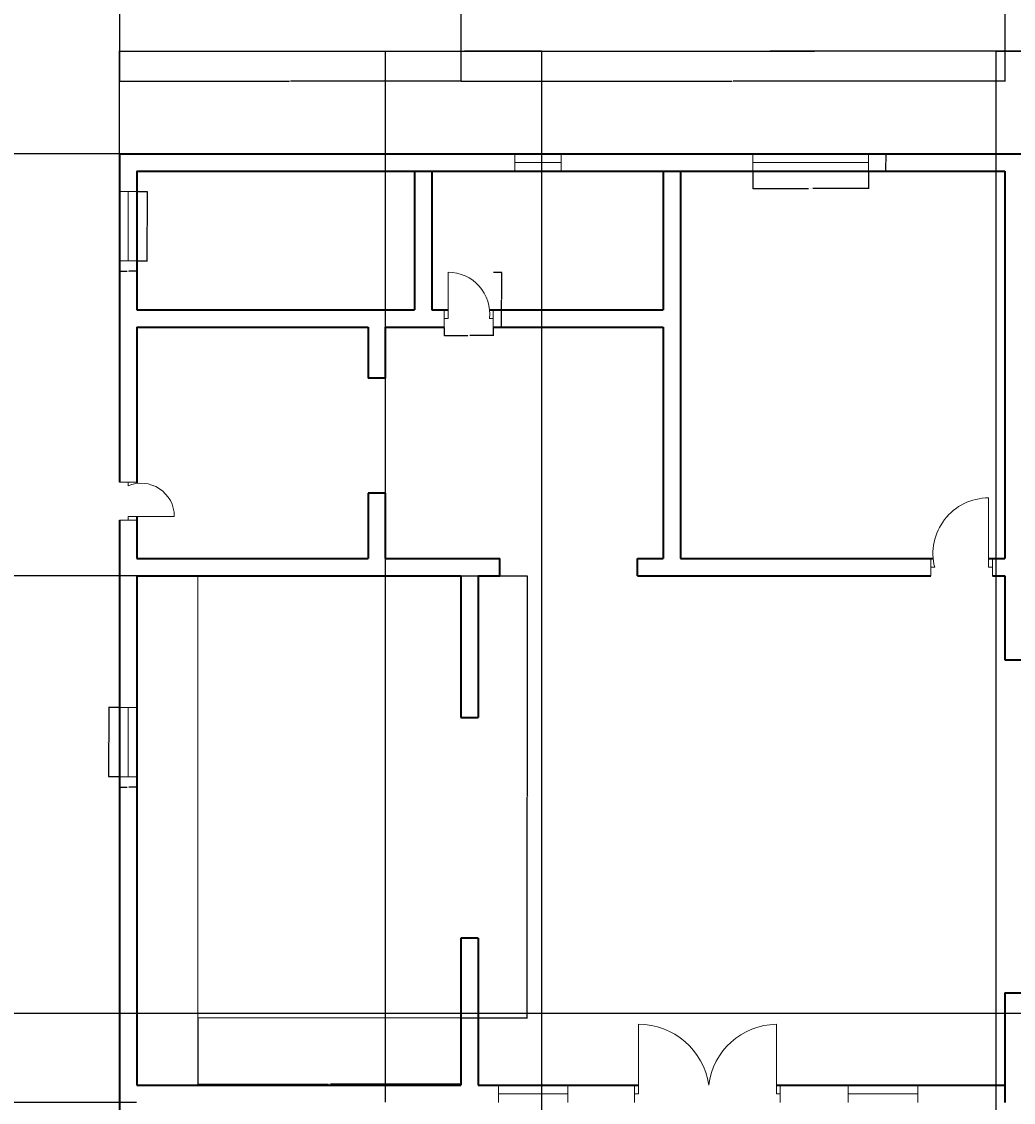
# Model space of a CAD drawing. Units: inches. Extents: x 2185 to 4426, y 1138 to 3073.
# Tile 11 of 14: x 3160 to 3674, y 1834 to 2395. Entities that reach past the tile are written whole.
import ezdxf

# ---------------------------------------------------------------- set-up
doc = ezdxf.new("R2010")
doc.units = ezdxf.units.IN
for name, color, linetype, lineweight in [('A-ANNO-DIMS', 2, 'Continuous', 18), ('A-ANNO-SYMB', 2, 'Continuous', 25), ('A-DOOR', 3, 'Continuous', 18), ('A-FLOR-CASE', 32, 'Continuous', 18), ('A-GLAZ', 4, 'Continuous', 18), ('A-WALL', 7, 'Continuous', 35)]:
    doc.layers.add(name, color=color, linetype=linetype, lineweight=lineweight)
doc.styles.get("Standard").update_dxf_attribs({"font": 'arial.ttf'})
doc.dimstyles.get("Standard").update_dxf_attribs({"dimtxt": 0.18, "dimasz": 0.18, "dimexe": 0.18, "dimexo": 0.0625, "dimgap": 0.09, "dimtad": 0, "dimtih": 1, "dimtoh": 1, "dimdec": 4, "dimzin": 0, "dimdsep": 46, "dimtxsty": 'Standard', "dimcen": 0.09, "dimadec": 0, "dimazin": 0, "dimtfac": 1, "dimtdec": 4, "dimtofl": 0, "dimtmove": 0, "dimatfit": 3, "dimfxl": 1, "dimtolj": 1, "dimtzin": 0, "dimarcsym": 0})

# ---------------------------------------------------------------- blocks, each defined once
blk = doc.blocks.new('DOOR-SGL-36-BED-W')
for p, q in [((29.94, 4.5), (29.94, 40.5)), ((0, 9), (0, 0)), ((31.94, 0), (31.94, 9)), ((31.94, 9), (31.94, 4.5)), ((0, 0), (0, 4.5)), ((0, 4.5), (2, 4.5)), ((31.94, 4.5), (29.94, 4.5)), ((0, 0), (0, 0))]:
    blk.add_line(p, q)
blk.add_arc((29.94, 11.66), 28.84, 90, 194.3796)
blk = doc.blocks.new('DOOR-SGL-24-STORE')
for p, q in [((2, 4.5), (2, 28.5)), ((0, 9), (0, 0)), ((25.41, 9), (25.41, 0)), ((0, 0), (0, 4.5)), ((0, 4.5), (2, 4.5)), ((25.41, 4.5), (23.41, 4.5)), ((25.41, 0), (25.41, 4.5))]:
    blk.add_line(p, q)
blk.add_arc((2, 6.95), 21.55, 353.479, 90)
blk = doc.blocks.new('DOOR-SGL-24-WORK')
for p, q in [((9, 19.77), (0, 19.77)), ((0, 19.77), (4.5, 19.77)), ((4.5, 19.77), (4.5, 17.77)), ((9, 0), (0, 0)), ((0, 0), (4.5, 0)), ((4.5, 0), (4.5, 2)), ((4.5, 2), (28.5, 2))]:
    blk.add_line(p, q)
blk.add_arc((11.32, 2), 17.18, 0, 113.3778)
blk = doc.blocks.new('DOOR-PAIR-36-DINING')
for p, q in [((2, 4.5), (2, 40.5)), ((73.51, 4.5), (73.51, 40.5)), ((0, 9), (0, 0)), ((75.51, 0), (75.51, 9)), ((75.51, 9), (75.51, 4.5)), ((0, 0), (0, 4.5)), ((0, 4.5), (2, 4.5)), ((75.51, 4.5), (73.51, 4.5))]:
    blk.add_line(p, q)
for centre, radius, start, end in [((2, 3.7), 36.8, 8.2761, 90), ((74.14, 4.5), 36.01, 90.9934, 172.8203)]:
    blk.add_arc(centre, radius, start, end)
blk = doc.blocks.new('WIN-PLAN-24IN-01')
for p, q in [((0, 9), (0, 0)), ((24, 4.5), (24, 9)), ((24, 9), (24, 0)), ((0, 0), (0, 4.5)), ((0, 4.5), (0, 4.5)), ((0, 4.5), (24, 4.5))]:
    blk.add_line(p, q)
blk = doc.blocks.new('WIN-PLAN-36IN-01')
for p, q in [((0, 9), (0, 0)), ((36, 4.5), (36, 9)), ((36, 9), (36, 0)), ((0, 0), (0, 4.5)), ((0, 4.5), (0, 4.5)), ((0, 4.5), (36, 4.5))]:
    blk.add_line(p, q)
blk = doc.blocks.new('WIN-PLAN-36IN-02')
for p, q in [((9, 36), (0, 36)), ((0, 36), (4.5, 36)), ((4.5, 36), (4.5, 0)), ((9, 0), (0, 0)), ((4.5, 0), (9, 0))]:
    blk.add_line(p, q)
blk = doc.blocks.new('WIN-PLAN-60IN-02')
for p, q in [((0, 9), (0, 0)), ((60, 4.5), (60, 9)), ((60, 9), (60, 0)), ((0, 0), (0, 4.5)), ((0, 4.5), (0, 4.5)), ((0, 4.5), (60, 4.5)), ((0, 0), (0, 0))]:
    blk.add_line(p, q)
blk = doc.blocks.new('KITCHEN-COUNTER-L')
for p, q in [((0, 0), (0, 229.1)), ((136.38, 0), (0, 0)), ((136.38, 0), (136.38, 0))]:
    blk.add_line(p, q)
blk = doc.blocks.new('*D56')
at = {"layer": 'A-ANNO-DIMS', "color": 0, "lineweight": -2, "transparency": 16777216}
for p, q in [((3210.79, 2039.2), (3205.27, 2039.2)), ((3205.45, 2039.02), (3205.45, 2021.38)), ((3205.45, 2003.38), (3205.45, 2021.02)), ((3210.79, 2003.2), (3205.27, 2003.2))]:
    blk.add_line(p, q, dxfattribs=at)
at = {"layer": 'A-ANNO-DIMS', "color": 0, "transparency": 16777216}
for points in [[(3205.42, 2039.02), (3205.48, 2039.02), (3205.45, 2039.2)], [(3205.42, 2003.38), (3205.48, 2003.38), (3205.45, 2003.2)]]:
    blk.add_solid(points, dxfattribs=at)
at = {"layer": 'Defpoints', "color": 0, "transparency": 16777216}
for p in [(3210.85, 2039.2), (3205.45, 2003.2), (3210.85, 2003.2)]:
    blk.add_point(p, dxfattribs=at)
at = {"layer": 'A-ANNO-DIMS', "color": 0, "transparency": 16777216, "insert": (3205.45, 2021.2), "char_height": 0.18, "attachment_point": 5}
blk.add_mtext('\\A1;WINDOW 36 TYP.', dxfattribs=at)
blk = doc.blocks.new('*D57')
at = {"layer": 'A-ANNO-DIMS', "color": 0, "lineweight": -2, "transparency": 16777216}
for p, q in [((3210.85, 2003.14), (3210.85, 1997.62)), ((3219.85, 2003.14), (3219.85, 1997.62)), ((3211.03, 1997.8), (3214.89, 1997.8)), ((3219.67, 1997.8), (3215.81, 1997.8))]:
    blk.add_line(p, q, dxfattribs=at)
at = {"layer": 'A-ANNO-DIMS', "color": 0, "transparency": 16777216}
for points in [[(3211.03, 1997.83), (3211.03, 1997.77), (3210.85, 1997.8)], [(3219.67, 1997.83), (3219.67, 1997.77), (3219.85, 1997.8)]]:
    blk.add_solid(points, dxfattribs=at)
at = {"layer": 'Defpoints', "color": 0, "transparency": 16777216}
for p in [(3210.85, 2003.2), (3219.85, 2003.2), (3219.85, 1997.8)]:
    blk.add_point(p, dxfattribs=at)
at = {"layer": 'A-ANNO-DIMS', "color": 0, "transparency": 16777216, "insert": (3215.35, 1997.8), "char_height": 0.18, "attachment_point": 5}
blk.add_mtext('\\A1;9 TYP.', dxfattribs=at)
blk = doc.blocks.new('*D58')
at = {"layer": 'A-ANNO-DIMS', "color": 0, "lineweight": -2, "transparency": 16777216}
for p, q in [((3219.91, 2306.86), (3225.43, 2306.86)), ((3225.25, 2306.68), (3225.25, 2289.05)), ((3225.25, 2271.04), (3225.25, 2288.68)), ((3219.91, 2270.86), (3225.43, 2270.86))]:
    blk.add_line(p, q, dxfattribs=at)
at = {"layer": 'A-ANNO-DIMS', "color": 0, "transparency": 16777216}
for points in [[(3225.22, 2306.68), (3225.28, 2306.68), (3225.25, 2306.86)], [(3225.22, 2271.04), (3225.28, 2271.04), (3225.25, 2270.86)]]:
    blk.add_solid(points, dxfattribs=at)
at = {"layer": 'Defpoints', "color": 0, "transparency": 16777216}
for p in [(3219.85, 2306.86), (3225.25, 2306.86), (3219.85, 2270.86)]:
    blk.add_point(p, dxfattribs=at)
at = {"layer": 'A-ANNO-DIMS', "color": 0, "transparency": 16777216, "insert": (3225.25, 2288.86), "char_height": 0.18, "attachment_point": 5}
blk.add_mtext('\\A1;WINDOW 36 TYP.', dxfattribs=at)
blk = doc.blocks.new('*D59')
at = {"layer": 'A-ANNO-DIMS', "color": 0, "lineweight": -2, "transparency": 16777216}
for p, q in [((3210.85, 2270.8), (3210.85, 2265.28)), ((3219.85, 2270.8), (3219.85, 2265.28)), ((3211.03, 2265.46), (3214.89, 2265.46)), ((3219.67, 2265.46), (3215.81, 2265.46))]:
    blk.add_line(p, q, dxfattribs=at)
at = {"layer": 'A-ANNO-DIMS', "color": 0, "transparency": 16777216}
for points in [[(3211.03, 2265.49), (3211.03, 2265.43), (3210.85, 2265.46)], [(3219.67, 2265.49), (3219.67, 2265.43), (3219.85, 2265.46)]]:
    blk.add_solid(points, dxfattribs=at)
at = {"layer": 'Defpoints', "color": 0, "transparency": 16777216}
for p in [(3210.85, 2270.86), (3219.85, 2270.86), (3219.85, 2265.46)]:
    blk.add_point(p, dxfattribs=at)
at = {"layer": 'A-ANNO-DIMS', "color": 0, "transparency": 16777216, "insert": (3215.35, 2265.46), "char_height": 0.18, "attachment_point": 5}
blk.add_mtext('\\A1;9 TYP.', dxfattribs=at)
blk = doc.blocks.new('*D68')
at = {"layer": 'A-ANNO-DIMS', "color": 0, "lineweight": -2, "transparency": 16777216}
for p, q in [((3404.8, 2264.88), (3409.19, 2264.88)), ((3409.01, 2264.7), (3409.01, 2250.81)), ((3409.01, 2236.56), (3409.01, 2250.44)), ((3404.8, 2236.38), (3409.19, 2236.38))]:
    blk.add_line(p, q, dxfattribs=at)
at = {"layer": 'A-ANNO-DIMS', "color": 0, "transparency": 16777216}
for points in [[(3408.98, 2264.7), (3409.04, 2264.7), (3409.01, 2264.88)], [(3408.98, 2236.56), (3409.04, 2236.56), (3409.01, 2236.38)]]:
    blk.add_solid(points, dxfattribs=at)
at = {"layer": 'Defpoints', "color": 0, "transparency": 16777216}
for p in [(3404.73, 2264.88), (3409.01, 2264.88), (3404.73, 2236.38)]:
    blk.add_point(p, dxfattribs=at)
at = {"layer": 'A-ANNO-DIMS', "color": 0, "transparency": 16777216, "insert": (3409.01, 2250.63), "char_height": 0.18, "attachment_point": 5}
blk.add_mtext('\\A1;DOOR 29 TYP.', dxfattribs=at)
blk = doc.blocks.new('*D69')
at = {"layer": 'A-ANNO-DIMS', "color": 0, "lineweight": -2, "transparency": 16777216}
for p, q in [((3379.32, 2236.31), (3379.32, 2231.92)), ((3379.5, 2232.1), (3391.5, 2232.1)), ((3404.55, 2232.1), (3392.56, 2232.1)), ((3404.73, 2236.31), (3404.73, 2231.92))]:
    blk.add_line(p, q, dxfattribs=at)
at = {"layer": 'A-ANNO-DIMS', "color": 0, "transparency": 16777216}
for points in [[(3379.5, 2232.13), (3379.5, 2232.07), (3379.32, 2232.1)], [(3404.55, 2232.13), (3404.55, 2232.07), (3404.73, 2232.1)]]:
    blk.add_solid(points, dxfattribs=at)
at = {"layer": 'Defpoints', "color": 0, "transparency": 16777216}
for p in [(3379.32, 2236.38), (3404.73, 2236.38), (3404.73, 2232.1)]:
    blk.add_point(p, dxfattribs=at)
at = {"layer": 'A-ANNO-DIMS', "color": 0, "transparency": 16777216, "insert": (3392.03, 2232.1), "char_height": 0.18, "attachment_point": 5}
blk.add_mtext('\\A1;25 TYP.', dxfattribs=at)
blk = doc.blocks.new('*D106')
at = {"layer": 'A-ANNO-DIMS', "color": 0, "lineweight": -2, "transparency": 16777216}
for p, q in [((3539.31, 2317.31), (3539.31, 2308.2)), ((3599.31, 2317.31), (3599.31, 2308.2)), ((3539.49, 2308.38), (3568.19, 2308.38)), ((3599.13, 2308.38), (3570.43, 2308.38))]:
    blk.add_line(p, q, dxfattribs=at)
at = {"layer": 'A-ANNO-DIMS', "color": 0, "transparency": 16777216}
for points in [[(3539.49, 2308.41), (3539.49, 2308.35), (3539.31, 2308.38)], [(3599.13, 2308.41), (3599.13, 2308.35), (3599.31, 2308.38)]]:
    blk.add_solid(points, dxfattribs=at)
at = {"layer": 'Defpoints', "color": 0, "transparency": 16777216}
for p in [(3539.31, 2317.38), (3599.31, 2317.38), (3599.31, 2308.38)]:
    blk.add_point(p, dxfattribs=at)
at = {"layer": 'A-ANNO-DIMS', "color": 0, "transparency": 16777216, "insert": (3569.31, 2308.38), "char_height": 0.18, "attachment_point": 5}
blk.add_mtext('\\A1;WINDOW 60 TYP.', dxfattribs=at)
blk = doc.blocks.new('*D107')
at = {"layer": 'A-ANNO-DIMS', "color": 0, "lineweight": -2, "transparency": 16777216}
for p, q in [((3599.37, 2326.38), (3608.49, 2326.38)), ((3608.31, 2326.2), (3608.31, 2322.06)), ((3608.31, 2317.56), (3608.31, 2321.7)), ((3599.37, 2317.38), (3608.49, 2317.38))]:
    blk.add_line(p, q, dxfattribs=at)
at = {"layer": 'A-ANNO-DIMS', "color": 0, "transparency": 16777216}
for points in [[(3608.28, 2326.2), (3608.34, 2326.2), (3608.31, 2326.38)], [(3608.28, 2317.56), (3608.34, 2317.56), (3608.31, 2317.38)]]:
    blk.add_solid(points, dxfattribs=at)
at = {"layer": 'Defpoints', "color": 0, "transparency": 16777216}
for p in [(3599.31, 2326.38), (3608.31, 2326.38), (3599.31, 2317.38)]:
    blk.add_point(p, dxfattribs=at)
at = {"layer": 'A-ANNO-DIMS', "color": 0, "transparency": 16777216, "insert": (3608.31, 2321.88), "char_height": 0.18, "attachment_point": 5}
blk.add_mtext('\\A1;9 TYP.', dxfattribs=at)
blk = doc.blocks.new('*D120')
at = {"layer": 'A-ANNO-DIMS', "color": 0, "lineweight": -2, "transparency": 16777216}
for p, q in [((3387.91, 2107.38), (3422.39, 2107.38)), ((3422.21, 2107.2), (3422.21, 1993.01)), ((3422.21, 1878.45), (3422.21, 1992.64)), ((3387.91, 1878.27), (3422.39, 1878.27))]:
    blk.add_line(p, q, dxfattribs=at)
at = {"layer": 'A-ANNO-DIMS', "color": 0, "transparency": 16777216}
for points in [[(3422.18, 2107.2), (3422.24, 2107.2), (3422.21, 2107.38)], [(3422.18, 1878.45), (3422.24, 1878.45), (3422.21, 1878.27)]]:
    blk.add_solid(points, dxfattribs=at)
at = {"layer": 'Defpoints', "color": 0, "transparency": 16777216}
for p in [(3387.85, 2107.38), (3422.21, 2107.38), (3387.85, 1878.27)]:
    blk.add_point(p, dxfattribs=at)
at = {"layer": 'A-ANNO-DIMS', "color": 0, "transparency": 16777216, "insert": (3422.21, 1992.82), "char_height": 0.18, "attachment_point": 5}
blk.add_mtext('\\A1;COUNTER 229 TYP.', dxfattribs=at)
blk = doc.blocks.new('*D121')
at = {"layer": 'A-ANNO-DIMS', "color": 0, "lineweight": -2, "transparency": 16777216}
for p, q in [((3251.47, 1878.21), (3251.47, 1843.73)), ((3387.85, 1878.21), (3387.85, 1843.73)), ((3251.65, 1843.91), (3319.07, 1843.91)), ((3387.67, 1843.91), (3320.25, 1843.91))]:
    blk.add_line(p, q, dxfattribs=at)
at = {"layer": 'A-ANNO-DIMS', "color": 0, "transparency": 16777216}
for points in [[(3251.65, 1843.94), (3251.65, 1843.88), (3251.47, 1843.91)], [(3387.67, 1843.94), (3387.67, 1843.88), (3387.85, 1843.91)]]:
    blk.add_solid(points, dxfattribs=at)
at = {"layer": 'Defpoints', "color": 0, "transparency": 16777216}
for p in [(3251.47, 1878.27), (3387.85, 1878.27), (3387.85, 1843.91)]:
    blk.add_point(p, dxfattribs=at)
at = {"layer": 'A-ANNO-DIMS', "color": 0, "transparency": 16777216, "insert": (3319.66, 1843.91), "char_height": 0.18, "attachment_point": 5}
blk.add_mtext('\\A1;136 TYP.', dxfattribs=at)
blk = doc.blocks.new('*D145')
at = {"layer": 'A-ANNO-DIMS', "color": 0, "lineweight": -2, "transparency": 16777216}
for p, q in [((3210.85, 2326.44), (3210.85, 2379.81)), ((3211.03, 2379.63), (3571.21, 2379.63)), ((3932.17, 2379.63), (3571.99, 2379.63)), ((3932.35, 2326.44), (3932.35, 2379.81))]:
    blk.add_line(p, q, dxfattribs=at)
at = {"layer": 'A-ANNO-DIMS', "color": 0, "transparency": 16777216}
for points in [[(3211.03, 2379.66), (3211.03, 2379.6), (3210.85, 2379.63)], [(3932.17, 2379.66), (3932.17, 2379.6), (3932.35, 2379.63)]]:
    blk.add_solid(points, dxfattribs=at)
at = {"layer": 'Defpoints', "color": 0, "transparency": 16777216}
for p in [(3932.35, 2379.63), (3210.85, 2326.38), (3932.35, 2326.38)]:
    blk.add_point(p, dxfattribs=at)
at = {"layer": 'A-ANNO-DIMS', "color": 0, "transparency": 16777216, "insert": (3571.6, 2379.63), "char_height": 0.18, "attachment_point": 5}
blk.add_mtext('\\A1;721.5', dxfattribs=at)
blk = doc.blocks.new('*D152')
at = {"layer": 'A-ANNO-DIMS', "color": 0, "lineweight": -2, "transparency": 16777216}
for p, q in [((3155.01, 1880.56), (3101.64, 1880.56)), ((3101.82, 1880.38), (3101.82, 1857.65)), ((3101.82, 1834.56), (3101.82, 1857.29)), ((3219.79, 1834.38), (3101.64, 1834.38))]:
    blk.add_line(p, q, dxfattribs=at)
at = {"layer": 'A-ANNO-DIMS', "color": 0, "transparency": 16777216}
for points in [[(3101.79, 1880.38), (3101.85, 1880.38), (3101.82, 1880.56)], [(3101.79, 1834.56), (3101.85, 1834.56), (3101.82, 1834.38)]]:
    blk.add_solid(points, dxfattribs=at)
at = {"layer": 'Defpoints', "color": 0, "transparency": 16777216}
for p in [(3101.82, 1880.56), (3155.07, 1880.56), (3219.85, 1834.38)]:
    blk.add_point(p, dxfattribs=at)
at = {"layer": 'A-ANNO-DIMS', "color": 0, "transparency": 16777216, "insert": (3101.82, 1857.47), "char_height": 0.18, "attachment_point": 5}
blk.add_mtext('\\A1;46.19', dxfattribs=at)
blk = doc.blocks.new('*D153')
at = {"layer": 'A-ANNO-DIMS', "color": 0, "lineweight": -2, "transparency": 16777216}
for p, q in [((3219.79, 2107.38), (3101.64, 2107.38)), ((3101.82, 2107.2), (3101.82, 1994.15)), ((3101.82, 1880.74), (3101.82, 1993.79)), ((3155.01, 1880.56), (3101.64, 1880.56))]:
    blk.add_line(p, q, dxfattribs=at)
at = {"layer": 'A-ANNO-DIMS', "color": 0, "transparency": 16777216}
for points in [[(3101.79, 2107.2), (3101.85, 2107.2), (3101.82, 2107.38)], [(3101.79, 1880.74), (3101.85, 1880.74), (3101.82, 1880.56)]]:
    blk.add_solid(points, dxfattribs=at)
at = {"layer": 'Defpoints', "color": 0, "transparency": 16777216}
for p in [(3101.82, 2107.38), (3219.85, 2107.38), (3155.07, 1880.56)]:
    blk.add_point(p, dxfattribs=at)
at = {"layer": 'A-ANNO-DIMS', "color": 0, "transparency": 16777216, "insert": (3101.82, 1993.97), "char_height": 0.18, "attachment_point": 5}
blk.add_mtext('\\A1;226.8', dxfattribs=at)
blk = doc.blocks.new('*D154')
at = {"layer": 'A-ANNO-DIMS', "color": 0, "lineweight": -2, "transparency": 16777216}
for p, q in [((3210.79, 2326.38), (3101.64, 2326.38)), ((3101.82, 2326.2), (3101.82, 2217.06)), ((3101.82, 2107.56), (3101.82, 2216.7)), ((3219.79, 2107.38), (3101.64, 2107.38))]:
    blk.add_line(p, q, dxfattribs=at)
at = {"layer": 'A-ANNO-DIMS', "color": 0, "transparency": 16777216}
for points in [[(3101.79, 2326.2), (3101.85, 2326.2), (3101.82, 2326.38)], [(3101.79, 2107.56), (3101.85, 2107.56), (3101.82, 2107.38)]]:
    blk.add_solid(points, dxfattribs=at)
at = {"layer": 'Defpoints', "color": 0, "transparency": 16777216}
for p in [(3101.82, 2326.38), (3210.85, 2326.38), (3219.85, 2107.38)]:
    blk.add_point(p, dxfattribs=at)
at = {"layer": 'A-ANNO-DIMS', "color": 0, "transparency": 16777216, "insert": (3101.82, 2216.88), "char_height": 0.18, "attachment_point": 5}
blk.add_mtext('\\A1;219', dxfattribs=at)
blk = doc.blocks.new('*D155')
at = {"layer": 'A-ANNO-DIMS', "color": 0, "lineweight": -2, "transparency": 16777216}
for p, q in [((3348.85, 1834.44), (3348.85, 2379.81)), ((3349.03, 2379.63), (3388.93, 2379.63)), ((3429.63, 2379.63), (3389.72, 2379.63)), ((3429.81, 1753.44), (3429.81, 2379.81))]:
    blk.add_line(p, q, dxfattribs=at)
at = {"layer": 'A-ANNO-DIMS', "color": 0, "transparency": 16777216}
for points in [[(3349.03, 2379.66), (3349.03, 2379.6), (3348.85, 2379.63)], [(3429.63, 2379.66), (3429.63, 2379.6), (3429.81, 2379.63)]]:
    blk.add_solid(points, dxfattribs=at)
at = {"layer": 'Defpoints', "color": 0, "transparency": 16777216}
for p in [(3429.81, 2379.63), (3348.85, 1834.38), (3429.81, 1753.38)]:
    blk.add_point(p, dxfattribs=at)
at = {"layer": 'A-ANNO-DIMS', "color": 0, "transparency": 16777216, "insert": (3389.33, 2379.63), "char_height": 0.18, "attachment_point": 5}
blk.add_mtext('\\A1;80.96', dxfattribs=at)
blk = doc.blocks.new('*D156')
at = {"layer": 'A-ANNO-DIMS', "color": 0, "lineweight": -2, "transparency": 16777216}
for p, q in [((3429.81, 1753.44), (3429.81, 2379.81)), ((3429.99, 2379.63), (3547.11, 2379.63)), ((3665.17, 2379.63), (3548.04, 2379.63)), ((3665.35, 1753.44), (3665.35, 2379.81))]:
    blk.add_line(p, q, dxfattribs=at)
at = {"layer": 'A-ANNO-DIMS', "color": 0, "transparency": 16777216}
for points in [[(3429.99, 2379.66), (3429.99, 2379.6), (3429.81, 2379.63)], [(3665.17, 2379.66), (3665.17, 2379.6), (3665.35, 2379.63)]]:
    blk.add_solid(points, dxfattribs=at)
at = {"layer": 'Defpoints', "color": 0, "transparency": 16777216}
for p in [(3665.35, 2379.63), (3429.81, 1753.38), (3665.35, 1753.38)]:
    blk.add_point(p, dxfattribs=at)
at = {"layer": 'A-ANNO-DIMS', "color": 0, "transparency": 16777216, "insert": (3547.58, 2379.63), "char_height": 0.18, "attachment_point": 5}
blk.add_mtext('\\A1;235.54', dxfattribs=at)
blk = doc.blocks.new('*D157')
at = {"layer": 'A-ANNO-DIMS', "color": 0, "lineweight": -2, "transparency": 16777216}
for p, q in [((3665.35, 1753.44), (3665.35, 2379.81)), ((3665.53, 2379.63), (3705.65, 2379.63)), ((3746.17, 2379.63), (3706.05, 2379.63)), ((3746.35, 1834.44), (3746.35, 2379.81))]:
    blk.add_line(p, q, dxfattribs=at)
at = {"layer": 'A-ANNO-DIMS', "color": 0, "transparency": 16777216}
for points in [[(3665.53, 2379.66), (3665.53, 2379.6), (3665.35, 2379.63)], [(3746.17, 2379.66), (3746.17, 2379.6), (3746.35, 2379.63)]]:
    blk.add_solid(points, dxfattribs=at)
at = {"layer": 'Defpoints', "color": 0, "transparency": 16777216}
for p in [(3746.35, 2379.63), (3746.35, 1834.38), (3665.35, 1753.38)]:
    blk.add_point(p, dxfattribs=at)
at = {"layer": 'A-ANNO-DIMS', "color": 0, "transparency": 16777216, "insert": (3705.85, 2379.63), "char_height": 0.18, "attachment_point": 5}
blk.add_mtext('\\A1;81', dxfattribs=at)
blk = doc.blocks.new('*D177')
at = {"layer": 'A-ANNO-DIMS', "color": 0, "lineweight": -2, "transparency": 16777216}
for p, q in [((3387.85, 2485.42), (3387.85, 2363.79)), ((3210.85, 2467.42), (3210.85, 2363.79)), ((3211.03, 2363.97), (3299.07, 2363.97)), ((3387.67, 2363.97), (3299.63, 2363.97))]:
    blk.add_line(p, q, dxfattribs=at)
at = {"layer": 'A-ANNO-DIMS', "color": 0, "transparency": 16777216}
for points in [[(3211.03, 2364), (3211.03, 2363.94), (3210.85, 2363.97)], [(3387.67, 2364), (3387.67, 2363.94), (3387.85, 2363.97)]]:
    blk.add_solid(points, dxfattribs=at)
at = {"layer": 'Defpoints', "color": 0, "transparency": 16777216}
for p in [(3387.85, 2485.48), (3210.85, 2467.48), (3387.85, 2363.97)]:
    blk.add_point(p, dxfattribs=at)
at = {"layer": 'A-ANNO-DIMS', "color": 0, "transparency": 16777216, "insert": (3299.35, 2363.97), "char_height": 0.18, "attachment_point": 5}
blk.add_mtext('\\A1;177', dxfattribs=at)
blk = doc.blocks.new('*D178')
at = {"layer": 'A-ANNO-DIMS', "color": 0, "lineweight": -2, "transparency": 16777216}
for p, q in [((3387.85, 2485.42), (3387.85, 2363.79)), ((3669.85, 2485.42), (3669.85, 2363.79)), ((3388.03, 2363.97), (3528.56, 2363.97)), ((3669.67, 2363.97), (3529.14, 2363.97))]:
    blk.add_line(p, q, dxfattribs=at)
at = {"layer": 'A-ANNO-DIMS', "color": 0, "transparency": 16777216}
for points in [[(3388.03, 2364), (3388.03, 2363.94), (3387.85, 2363.97)], [(3669.67, 2364), (3669.67, 2363.94), (3669.85, 2363.97)]]:
    blk.add_solid(points, dxfattribs=at)
at = {"layer": 'Defpoints', "color": 0, "transparency": 16777216}
for p in [(3387.85, 2485.48), (3669.85, 2485.48), (3669.85, 2363.97)]:
    blk.add_point(p, dxfattribs=at)
at = {"layer": 'A-ANNO-DIMS', "color": 0, "transparency": 16777216, "insert": (3528.85, 2363.97), "char_height": 0.18, "attachment_point": 5}
blk.add_mtext('\\A1;282', dxfattribs=at)

msp = doc.modelspace()

# ---------------------------------------------------------------- linework, layer by layer
at = {"layer": 'A-ANNO-SYMB'}
msp.add_line((3155.074, 1880.563), (4005.21, 1880.563), dxfattribs=at)
at = {"layer": 'A-WALL'}
for p, q in [((3210.849, 2326.377), (3210.849, 2156.075)), ((3210.849, 2326.377), (3210.849, 2156.075)), ((3210.849, 2326.377), (3932.349, 2326.377)), ((3210.849, 2326.377), (3210.849, 2156.075)), ((3210.849, 2326.377), (3210.849, 2156.075)), ((3210.849, 2326.377), (3932.349, 2326.377)), ((3219.849, 2317.377), (3219.849, 2245.377)), ((3219.849, 2317.377), (3669.849, 2317.377)), ((3219.849, 2317.377), (3219.849, 2245.377)), ((3219.849, 2317.377), (3669.849, 2317.377)), ((3363.849, 2317.377), (3363.849, 2245.377)), ((3363.849, 2317.377), (3363.849, 2245.377)), ((3372.849, 2317.377), (3372.849, 2245.377)), ((3372.849, 2317.377), (3372.849, 2245.377)), ((3492.849, 2317.377), (3492.849, 2245.377)), ((3492.849, 2317.377), (3492.849, 2245.377)), ((3501.849, 2317.377), (3501.849, 2116.377)), ((3501.849, 2317.377), (3501.849, 2116.377)), ((3669.849, 2317.377), (3669.849, 2116.377)), ((3669.849, 2317.377), (3669.849, 2116.377)), ((3219.849, 2245.377), (3363.849, 2245.377)), ((3219.849, 2245.377), (3363.849, 2245.377)), ((3372.849, 2245.377), (3381.32, 2245.377)), ((3372.849, 2245.377), (3381.32, 2245.377)), ((3402.775, 2245.377), (3492.849, 2245.377)), ((3402.775, 2245.377), (3492.849, 2245.377)), ((3219.849, 2236.377), (3219.849, 2155.328)), ((3219.849, 2236.377), (3339.849, 2236.377)), ((3219.849, 2236.377), (3339.849, 2236.377)), ((3219.849, 2236.377), (3219.849, 2155.328)), ((3219.849, 2236.377), (3339.849, 2236.377)), ((3219.849, 2236.377), (3339.849, 2236.377)), ((3339.849, 2236.377), (3339.849, 2209.971)), ((3339.849, 2236.377), (3339.849, 2209.971)), ((3348.849, 2236.377), (3372.849, 2236.377)), ((3348.849, 2209.971), (3348.849, 2236.377)), ((3348.849, 2236.377), (3372.849, 2236.377)), ((3348.849, 2209.971), (3348.849, 2236.377)), ((3372.849, 2236.377), (3379.32, 2236.377)), ((3372.849, 2236.377), (3379.32, 2236.377)), ((3404.733, 2236.377), (3492.849, 2236.377)), ((3404.733, 2236.377), (3492.849, 2236.377)), ((3492.849, 2236.377), (3492.849, 2116.377)), ((3492.849, 2236.377), (3492.849, 2116.377)), ((3348.849, 2209.971), (3339.849, 2209.971)), ((3348.849, 2209.971), (3339.849, 2209.971)), ((3339.849, 2150.249), (3339.849, 2116.377)), ((3348.849, 2150.249), (3339.849, 2150.249)), ((3339.849, 2150.249), (3339.849, 2116.377)), ((3348.849, 2150.249), (3339.849, 2150.249)), ((3348.849, 2116.377), (3348.849, 2150.249)), ((3348.849, 2116.377), (3348.849, 2150.249)), ((3210.849, 2136.303), (3210.849, 1327.377)), ((3210.849, 2136.303), (3210.849, 1327.377)), ((3210.849, 2136.303), (3210.849, 1327.377)), ((3210.849, 2136.303), (3210.849, 1327.377)), ((3219.849, 2138.303), (3219.849, 2116.377)), ((3219.849, 2138.303), (3219.849, 2116.377)), ((3219.849, 2116.377), (3339.849, 2116.377)), ((3219.849, 2116.377), (3339.849, 2116.377)), ((3348.849, 2116.377), (3372.849, 2116.377)), ((3348.849, 2116.377), (3372.849, 2116.377)), ((3372.849, 2116.377), (3408.138, 2116.377)), ((3372.849, 2116.377), (3408.138, 2116.377)), ((3408.138, 2107.377), (3408.138, 2116.377)), ((3408.138, 2107.377), (3408.138, 2116.377)), ((3479.415, 2116.377), (3492.849, 2116.377)), ((3479.415, 2107.377), (3479.415, 2116.377)), ((3479.415, 2116.377), (3492.849, 2116.377)), ((3479.415, 2107.377), (3479.415, 2116.377)), ((3501.849, 2116.377), (3632.773, 2116.377)), ((3501.849, 2116.377), (3632.773, 2116.377)), ((3661.488, 2116.377), (3669.849, 2116.377)), ((3661.488, 2116.377), (3669.849, 2116.377)), ((3219.849, 2107.377), (3219.849, 1843.377)), ((3219.849, 2107.377), (3363.849, 2107.377)), ((3219.849, 2107.377), (3219.849, 1843.377)), ((3219.849, 2107.377), (3363.849, 2107.377)), ((3363.849, 2107.377), (3387.849, 2107.377)), ((3363.849, 2107.377), (3387.849, 2107.377)), ((3387.849, 2107.377), (3387.849, 2033.934)), ((3387.849, 2107.377), (3387.849, 2033.934)), ((3396.849, 2107.377), (3396.849, 2033.934)), ((3396.849, 2107.377), (3408.138, 2107.377)), ((3396.849, 2107.377), (3396.849, 2033.934)), ((3396.849, 2107.377), (3408.138, 2107.377)), ((3479.415, 2107.377), (3631.553, 2107.377)), ((3479.415, 2107.377), (3631.553, 2107.377)), ((3663.488, 2107.377), (3669.849, 2107.377)), ((3663.488, 2107.377), (3669.849, 2107.377)), ((3669.849, 2107.377), (3669.849, 2063.852)), ((3669.849, 2107.377), (3669.849, 2063.852)), ((3669.849, 2063.852), (3678.849, 2063.852)), ((3669.849, 2063.852), (3678.849, 2063.852)), ((3387.849, 2033.934), (3396.849, 2033.934)), ((3387.849, 2033.934), (3396.849, 2033.934)), ((3387.849, 1919.604), (3387.849, 1843.377)), ((3396.849, 1919.604), (3387.849, 1919.604)), ((3387.849, 1919.604), (3387.849, 1843.377)), ((3396.849, 1919.604), (3387.849, 1919.604)), ((3396.849, 1919.604), (3396.849, 1843.377)), ((3396.849, 1919.604), (3396.849, 1843.377)), ((3219.849, 1906.377), (3219.849, 1843.377)), ((3219.849, 1906.377), (3219.849, 1843.377)), ((3669.849, 1891.155), (3669.849, 1843.377)), ((3669.849, 1891.155), (3678.849, 1891.155)), ((3669.849, 1891.155), (3669.849, 1843.377)), ((3669.849, 1891.155), (3678.849, 1891.155)), ((3219.849, 1843.377), (3363.849, 1843.377)), ((3219.849, 1843.377), (3363.849, 1843.377)), ((3363.849, 1843.377), (3387.849, 1843.377)), ((3363.849, 1843.377), (3387.849, 1843.377)), ((3396.849, 1843.377), (3479.974, 1843.377)), ((3396.849, 1843.377), (3479.974, 1843.377)), ((3551.486, 1843.377), (3669.849, 1843.377)), ((3551.486, 1843.377), (3669.849, 1843.377)), ((3669.849, 1843.377), (3669.849, 1834.377)), ((3669.849, 1843.377), (3669.849, 1834.377))]:
    msp.add_line(p, q, dxfattribs=at)

# ---------------------------------------------------------------- block references
at = {"layer": 'A-DOOR'}
for name, p in [('DOOR-SGL-24-STORE', (3379.32, 2236.377)), ('DOOR-SGL-24-STORE', (3379.32, 2236.377)), ('DOOR-SGL-24-WORK', (3210.849, 2136.303)), ('DOOR-SGL-24-WORK', (3210.849, 2136.303)), ('DOOR-SGL-36-BED-W', (3631.553, 2107.377)), ('DOOR-SGL-36-BED-W', (3631.553, 2107.377)), ('DOOR-PAIR-36-DINING', (3477.974, 1834.377)), ('DOOR-PAIR-36-DINING', (3477.974, 1834.377))]:
    msp.add_blockref(name, p, dxfattribs=at)
at = {"layer": 'A-FLOR-CASE'}
msp.add_blockref('KITCHEN-COUNTER-L', (3251.473, 1878.273), dxfattribs=at)
msp.add_blockref('KITCHEN-COUNTER-L', (3251.473, 1878.273), dxfattribs=at)
at = {"layer": 'A-GLAZ'}
for name, p in [('WIN-PLAN-24IN-01', (3415.886, 2317.377)), ('WIN-PLAN-24IN-01', (3415.886, 2317.377)), ('WIN-PLAN-60IN-02', (3539.312, 2317.377)), ('WIN-PLAN-60IN-02', (3539.312, 2317.377)), ('WIN-PLAN-36IN-02', (3210.849, 2270.862)), ('WIN-PLAN-36IN-02', (3210.849, 2270.862)), ('WIN-PLAN-36IN-01', (3588.761, 1834.377)), ('WIN-PLAN-36IN-01', (3588.761, 1834.377))]:
    msp.add_blockref(name, p, dxfattribs=at)
for name, p, rotation in [('WIN-PLAN-36IN-01', (3210.849, 2039.2), 270.0000000000025), ('WIN-PLAN-36IN-01', (3210.849, 2039.2), 270.0000000000025), ('WIN-PLAN-36IN-02', (3443.369, 1834.377), 90.00000000000102), ('WIN-PLAN-36IN-02', (3443.369, 1834.377), 90.00000000000102)]:
    msp.add_blockref(name, p, dxfattribs=dict(at, rotation=rotation))

# ---------------------------------------------------------------- dimensions: what is measured, and where the dimension line sits
at = {"layer": 'A-ANNO-DIMS'}
for base, p1, p2, override, picture, middle in [((3387.849, 2363.967), (3210.849, 2467.482), (3387.849, 2485.482), {"dimdec": 0, "dimlfac": 1, "dimrnd": 0, "dimzin": 0, "dimdsep": 46, "dimlunit": 2}, '*D177', (3299.349, 2363.967)), ((3669.849, 2363.967), (3387.849, 2485.482), (3669.849, 2485.482), {"dimdec": 0, "dimlfac": 1, "dimrnd": 0, "dimzin": 0, "dimdsep": 46, "dimlunit": 2}, '*D178', (3528.849, 2363.967)), ((3932.349, 2379.627), (3210.849, 2326.377), (3932.349, 2326.377), {"dimdec": 1, "dimlfac": 1, "dimrnd": 0, "dimzin": 0, "dimdsep": 46, "dimlunit": 2}, '*D145', (3571.599, 2379.627)), ((3429.807, 2379.627), (3348.849, 1834.377), (3429.807, 1753.377), {"dimdec": 2, "dimlfac": 1, "dimrnd": 0, "dimzin": 0, "dimdsep": 46, "dimlunit": 2}, '*D155', (3389.328, 2379.627)), ((3665.349, 2379.627), (3429.807, 1753.377), (3665.349, 1753.377), {"dimdec": 2, "dimlfac": 1, "dimrnd": 0, "dimzin": 0, "dimdsep": 46, "dimlunit": 2}, '*D156', (3547.578, 2379.627)), ((3746.349, 2379.627), (3665.349, 1753.377), (3746.349, 1834.377), {"dimdec": 0, "dimlfac": 1, "dimrnd": 0, "dimzin": 0, "dimdsep": 46, "dimlunit": 2}, '*D157', (3705.849, 2379.627))]:
    dim = msp.add_linear_dim(base=base, p1=p1, p2=p2, dimstyle='Standard', override=override, dxfattribs=at)
    dim.commit()
    dim.dimension.update_dxf_attribs({"geometry": picture, "text_midpoint": middle})
for base, p1, p2, override, picture, middle in [((3101.824, 2326.377), (3219.849, 2107.377), (3210.849, 2326.377), {"dimdec": 0, "dimlfac": 1, "dimrnd": 0, "dimzin": 0, "dimdsep": 46, "dimlunit": 2}, '*D154', (3101.824, 2216.877)), ((3101.824, 2107.377), (3155.074, 1880.563), (3219.849, 2107.377), {"dimdec": 1, "dimlfac": 1, "dimrnd": 0, "dimzin": 0, "dimdsep": 46, "dimlunit": 2}, '*D153', (3101.824, 1993.97)), ((3101.824, 1880.563), (3219.849, 1834.377), (3155.074, 1880.563), {"dimdec": 2, "dimlfac": 1, "dimrnd": 0, "dimzin": 0, "dimdsep": 46, "dimlunit": 2}, '*D152', (3101.824, 1857.47))]:
    dim = msp.add_linear_dim(base=base, p1=p1, p2=p2, angle=90, dimstyle='Standard', override=override, dxfattribs=at)
    dim.commit()
    dim.dimension.update_dxf_attribs({"geometry": picture, "text_midpoint": middle})
for base, p1, p2, angle, text, picture, middle in [((3608.311, 2326.377), (3599.311, 2317.377), (3599.311, 2326.377), 90, '<> TYP.', '*D107', (3608.311, 2321.877)), ((3225.249, 2306.862), (3219.849, 2270.862), (3219.849, 2306.862), 90, 'WINDOW <> TYP.', '*D58', (3225.249, 2288.862)), ((3409.008196256, 2264.876947079), (3404.733196256, 2236.376947079), (3404.733196256, 2264.876947079), 90, 'DOOR <> TYP.', '*D68', (3409.008196256, 2250.626947079)), ((3422.215, 2107.377), (3387.849, 1878.273), (3387.849, 2107.377), 90, 'COUNTER <> TYP.', '*D120', (3422.215, 1992.825)), ((3205.449, 2003.2), (3210.849, 2039.2), (3210.849, 2003.2), 270, 'WINDOW <> TYP.', '*D56', (3205.449, 2021.2)), ((3219.849, 1997.8), (3210.849, 2003.2), (3219.849, 2003.2), 0, '<> TYP.', '*D57', (3215.349, 1997.8))]:
    dim = msp.add_linear_dim(base=base, p1=p1, p2=p2, angle=angle, text=text, dimstyle='Standard', override={"dimdec": 0, "dimlfac": 1, "dimrnd": 0, "dimzin": 0, "dimdsep": 46, "dimlunit": 2}, dxfattribs=at)
    dim.commit()
    dim.dimension.update_dxf_attribs({"geometry": picture, "text_midpoint": middle})
for base, p1, p2, text, picture, middle in [((3599.311, 2308.377), (3539.311, 2317.377), (3599.311, 2317.377), 'WINDOW <> TYP.', '*D106', (3569.311, 2308.377)), ((3219.849, 2265.462), (3210.849, 2270.862), (3219.849, 2270.862), '<> TYP.', '*D59', (3215.349, 2265.462)), ((3404.733, 2232.102), (3379.32, 2236.377), (3404.733, 2236.377), '<> TYP.', '*D69', (3392.027, 2232.102)), ((3387.849, 1843.907), (3251.473, 1878.273), (3387.849, 1878.273), '<> TYP.', '*D121', (3319.661, 1843.907))]:
    dim = msp.add_linear_dim(base=base, p1=p1, p2=p2, text=text, dimstyle='Standard', override={"dimdec": 0, "dimlfac": 1, "dimrnd": 0, "dimzin": 0, "dimdsep": 46, "dimlunit": 2}, dxfattribs=at)
    dim.commit()
    dim.dimension.update_dxf_attribs({"geometry": picture, "text_midpoint": middle})

doc.saveas('drawing.dxf')
